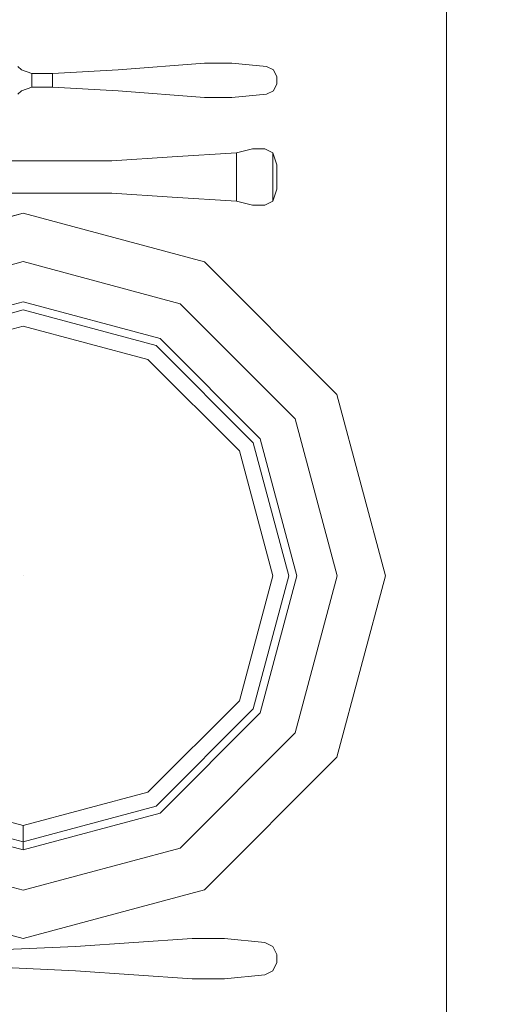
# Model space of a CAD drawing. Units: inches. Extents: x 375 to 1122, y 27 to 1069.
# Tile 63 of 155: x 739.72 to 747.02, y 296.54 to 311.59. Entities that reach past the tile are written whole.
import ezdxf

# ---------------------------------------------------------------- set-up
doc = ezdxf.new("R2010")
doc.units = ezdxf.units.IN
doc.layers.add('A-ANNO-DIMS', color=2, linetype='Continuous', lineweight=18)
doc.layers.add('Furniture', color=30, linetype='Continuous', lineweight=18)
doc.styles.get("Standard").update_dxf_attribs({"font": 'arial.ttf'})
doc.dimstyles.new('ISO-25', dxfattribs={"dimtxt": 12, "dimasz": 2.5, "dimexe": 1.5, "dimexo": 1.5, "dimtad": 1, "dimdec": 1, "dimlunit": 3, "dimtxsty": 'Standard', "dimblk": 'ARCHTICK', "dimcen": 2.5, "dimadec": 0, "dimazin": 0, "dimtfac": 1, "dimtdec": 1, "dimtmove": 0, "dimatfit": 3, "dimfxl": 1.5, "dimfxlon": 1, "dimarcsym": 0})

# ---------------------------------------------------------------- blocks, each defined once
blk = doc.blocks.new('A$C403C54AD')
blk.add_line((0.83575, 1.53256, -0.0006), (1.99923, 1.53256, -0.0006))
at = {"linetype": 'ByBlock'}
for points, invisible_edges in [([(1.0802, 1.50922, -0.02349), (1.0802, 1.49075, -0.02349), (1.02018, 1.47466, -0.02349), (1.01094, 1.49066, -0.02349)], 5), ([(1.0802, 1.47535, -0.03734), (1.0802, 1.50922, -0.02811), (1.01094, 1.49066, -0.02811), (1.02787, 1.46133, -0.03734)], 5), ([(1.14947, 1.49066, -0.02349), (1.14023, 1.47466, -0.02349), (1.0802, 1.49075, -0.02349), (1.0802, 1.50922, -0.02349)], 5), ([(1.13254, 1.46133, -0.03734), (1.14947, 1.49066, -0.02811), (1.0802, 1.50922, -0.02811), (1.0802, 1.47535, -0.03734)], 5), ([(1.01094, 1.49066, -0.02349), (1.02018, 1.47466, -0.02349), (0.97623, 1.43072, -0.02349), (0.96024, 1.43995, -0.02349)], 5), ([(1.02787, 1.46133, -0.03734), (1.01094, 1.49066, -0.02811), (0.96024, 1.43995, -0.02811), (0.98956, 1.42302, -0.03734)], 5), ([(1.0802, 1.49075, -0.02349), (1.0802, 1.47228, -0.02965), (1.02941, 1.45867, -0.02965), (1.02018, 1.47466, -0.02349)], 5), ([(1.14023, 1.47466, -0.02349), (1.131, 1.45867, -0.02965), (1.0802, 1.47228, -0.02965), (1.0802, 1.49075, -0.02349)], 5), ([(1.17085, 1.42302, -0.03734), (1.20017, 1.43995, -0.02811), (1.14947, 1.49066, -0.02811), (1.13254, 1.46133, -0.03734)], 5), ([(1.20017, 1.43995, -0.02349), (1.18418, 1.43072, -0.02349), (1.14023, 1.47466, -0.02349), (1.14947, 1.49066, -0.02349)], 5), ([(1.02018, 1.47466, -0.02349), (1.02941, 1.45867, -0.02965), (0.99223, 1.42148, -0.02965), (0.97623, 1.43072, -0.02349)], 5), ([(1.0802, 1.46612, -0.04658), (1.0802, 1.47535, -0.03734), (1.02787, 1.46133, -0.03734), (1.03249, 1.45333, -0.04658)], 5), ([(1.12792, 1.45333, -0.04658), (1.13254, 1.46133, -0.03734), (1.0802, 1.47535, -0.03734), (1.0802, 1.46612, -0.04658)], 5), ([(1.18418, 1.43072, -0.02349), (1.16818, 1.42148, -0.02965), (1.131, 1.45867, -0.02965), (1.14023, 1.47466, -0.02349)], 5), ([(1.0802, 1.47228, -0.02965), (1.0802, 1.37069, -0.02965), (1.0802, 1.37069, -0.02965), (1.02941, 1.45867, -0.02965)], 5), ([(1.131, 1.45867, -0.02965), (1.0802, 1.37069, -0.02965), (1.0802, 1.37069, -0.02965), (1.0802, 1.47228, -0.02965)], 5), ([(1.03249, 1.45333, -0.04658), (1.02787, 1.46133, -0.03734), (0.98956, 1.42302, -0.03734), (0.99756, 1.4184, -0.04658)], 5), ([(1.16285, 1.4184, -0.04658), (1.17085, 1.42302, -0.03734), (1.13254, 1.46133, -0.03734), (1.12792, 1.45333, -0.04658)], 5), ([(1.02941, 1.45867, -0.02965), (1.0802, 1.37069, -0.02965), (1.0802, 1.37069, -0.02965), (0.99223, 1.42148, -0.02965)], 5), ([(1.16818, 1.42148, -0.02965), (1.0802, 1.37069, -0.02965), (1.0802, 1.37069, -0.02965), (1.131, 1.45867, -0.02965)], 5), ([(0.96024, 1.43995, -0.02349), (0.97623, 1.43072, -0.02349), (0.96015, 1.37069, -0.02349), (0.94168, 1.37069, -0.02349)], 5), ([(0.98956, 1.42302, -0.03734), (0.96024, 1.43995, -0.02811), (0.94168, 1.37069, -0.02811), (0.97554, 1.37069, -0.03734)], 5), ([(1.18487, 1.37069, -0.03734), (1.21873, 1.37069, -0.02811), (1.20017, 1.43995, -0.02811), (1.17085, 1.42302, -0.03734)], 5), ([(1.21873, 1.37069, -0.02349), (1.20026, 1.37069, -0.02349), (1.18418, 1.43072, -0.02349), (1.20017, 1.43995, -0.02349)], 5), ([(0.97623, 1.43072, -0.02349), (0.99223, 1.42148, -0.02965), (0.97862, 1.37069, -0.02965), (0.96015, 1.37069, -0.02349)], 5), ([(1.20026, 1.37069, -0.02349), (1.18179, 1.37069, -0.02965), (1.16818, 1.42148, -0.02965), (1.18418, 1.43072, -0.02349)], 5), ([(0.99756, 1.4184, -0.04658), (0.98956, 1.42302, -0.03734), (0.97554, 1.37069, -0.03734), (0.98477, 1.37069, -0.04658)], 5), ([(1.17563, 1.37069, -0.04658), (1.18487, 1.37069, -0.03734), (1.17085, 1.42302, -0.03734), (1.16285, 1.4184, -0.04658)], 4), ([(0.99223, 1.42148, -0.02965), (1.0802, 1.37069, -0.02965), (1.0802, 1.37069, -0.02965), (0.97862, 1.37069, -0.02965)], 5), ([(1.18179, 1.37069, -0.02965), (1.0802, 1.37069, -0.02965), (1.0802, 1.37069, -0.02965), (1.16818, 1.42148, -0.02965)], 5), ([(0.94168, 1.37069, -0.02349), (0.96015, 1.37069, -0.02349), (0.97623, 1.31066, -0.02349), (0.96024, 1.30143, -0.02349)], 5), ([(0.97554, 1.37069, -0.03734), (0.94168, 1.37069, -0.02811), (0.96024, 1.30143, -0.02811), (0.98956, 1.31836, -0.03734)], 5), ([(0.96015, 1.37069, -0.02349), (0.97862, 1.37069, -0.02965), (0.99223, 1.3199, -0.02965), (0.97623, 1.31066, -0.02349)], 5), ([(0.98477, 1.37069, -0.04658), (0.97554, 1.37069, -0.03734), (0.98956, 1.31836, -0.03734), (0.99756, 1.32297, -0.04658)], 5), ([(0.97862, 1.37069, -0.02965), (1.0802, 1.37069, -0.02965), (1.0802, 1.37069, -0.02965), (0.99223, 1.3199, -0.02965)], 5), ([(0.99223, 1.3199, -0.02965), (1.0802, 1.37069, -0.02965), (1.0802, 1.37069, -0.02965), (1.02941, 1.28271, -0.02965)], 5), ([(1.02941, 1.28271, -0.02965), (1.0802, 1.37069, -0.02965), (1.0802, 1.37069, -0.02965), (1.0802, 1.2691, -0.02965)], 5), ([(1.0802, 1.2691, -0.02965), (1.0802, 1.37069, -0.02965), (1.0802, 1.37069, -0.02965), (1.131, 1.28271, -0.02965)], 5), ([(1.16818, 1.3199, -0.02965), (1.0802, 1.37069, -0.02965), (1.0802, 1.37069, -0.02965), (1.18179, 1.37069, -0.02965)], 5), ([(1.131, 1.28271, -0.02965), (1.0802, 1.37069, -0.02965), (1.0802, 1.37069, -0.02965), (1.16818, 1.3199, -0.02965)], 5), ([(1.18418, 1.31066, -0.02349), (1.16818, 1.3199, -0.02965), (1.18179, 1.37069, -0.02965), (1.20026, 1.37069, -0.02349)], 5), ([(1.17085, 1.31836, -0.03734), (1.20017, 1.30143, -0.02811), (1.21873, 1.37069, -0.02811), (1.18487, 1.37069, -0.03734)], 5), ([(1.20017, 1.30143, -0.02349), (1.18418, 1.31066, -0.02349), (1.20026, 1.37069, -0.02349), (1.21873, 1.37069, -0.02349)], 5)]:
    blk.add_3dface(points, dxfattribs=dict(at, invisible_edges=invisible_edges))
for points in [[(1.0802, 1.50922, -0.02811), (1.0802, 1.50922, -0.02349), (1.01094, 1.49066, -0.02349), (1.01094, 1.49066, -0.02811)], [(1.14947, 1.49066, -0.02811), (1.14947, 1.49066, -0.02349), (1.0802, 1.50922, -0.02349), (1.0802, 1.50922, -0.02811)], [(1.01094, 1.49066, -0.02811), (1.01094, 1.49066, -0.02349), (0.96024, 1.43995, -0.02349), (0.96024, 1.43995, -0.02811)], [(1.20017, 1.43995, -0.02811), (1.20017, 1.43995, -0.02349), (1.14947, 1.49066, -0.02349), (1.14947, 1.49066, -0.02811)], [(0.96024, 1.43995, -0.02811), (0.96024, 1.43995, -0.02349), (0.94168, 1.37069, -0.02349), (0.94168, 1.37069, -0.02811)], [(1.21873, 1.37069, -0.02811), (1.21873, 1.37069, -0.02349), (1.20017, 1.43995, -0.02349), (1.20017, 1.43995, -0.02811)], [(0.94168, 1.37069, -0.02811), (0.94168, 1.37069, -0.02349), (0.96024, 1.30143, -0.02349), (0.96024, 1.30143, -0.02811)], [(1.16285, 1.32297, -0.04658), (1.17085, 1.31836, -0.03734), (1.18487, 1.37069, -0.03734), (1.17563, 1.37069, -0.04658)], [(1.20017, 1.30143, -0.02811), (1.20017, 1.30143, -0.02349), (1.21873, 1.37069, -0.02349), (1.21873, 1.37069, -0.02811)]]:
    blk.add_3dface(points, dxfattribs=at)
for points, invisible_edges in [([(0.8922, 1.46766, -0.04251), (0.88956, 1.46766, -0.04251), (0.88693, 1.46634, -0.04237), (0.89484, 1.46634, -0.04237)], 4), ([(0.8922, 1.46766, -0.04605), (0.88956, 1.46766, -0.04605), (0.88693, 1.46634, -0.04634), (0.89484, 1.46634, -0.04634)], 4), ([(1.22797, 1.46766, -0.03413), (1.22489, 1.46766, -0.03413), (1.22181, 1.46612, -0.03397), (1.23105, 1.46612, -0.03397)], 4), ([(1.22797, 1.46766, -0.03827), (1.22489, 1.46766, -0.03827), (1.22181, 1.46612, -0.0386), (1.23105, 1.46612, -0.0386)], 4), ([(0.89616, 1.4637, -0.04257), (0.88561, 1.4637, -0.04257), (0.88429, 1.45051, -0.0426), (0.89748, 1.45051, -0.0426)], 5), ([(0.89616, 1.4637, -0.04655), (0.88561, 1.4637, -0.04655), (0.88429, 1.45051, -0.04658), (0.89748, 1.45051, -0.04658)], 5), ([(0.88693, 1.46634, -0.04237), (0.89484, 1.46634, -0.04237), (0.89616, 1.4637, -0.04257), (0.88561, 1.4637, -0.04257)], 5), ([(0.88693, 1.46634, -0.04634), (0.89484, 1.46634, -0.04634), (0.89616, 1.4637, -0.04655), (0.88561, 1.4637, -0.04655)], 5), ([(0.91705, 1.46304, -0.03581), (0.9386, 1.46304, -0.03581), (0.93706, 1.46612, -0.03734), (0.91859, 1.46612, -0.03734)], 1), ([(0.91705, 1.46304, -0.04504), (0.9386, 1.46304, -0.04504), (0.93706, 1.46612, -0.0435), (0.91859, 1.46612, -0.0435)], 1), ([(1.22181, 1.46612, -0.03397), (1.23105, 1.46612, -0.03397), (1.23258, 1.46304, -0.03421), (1.22027, 1.46304, -0.03421)], 5), ([(1.22181, 1.46612, -0.0386), (1.23105, 1.46612, -0.0386), (1.23258, 1.46304, -0.03884), (1.22027, 1.46304, -0.03884)], 5), ([(0.9386, 1.45842, -0.03427), (0.91705, 1.45842, -0.03427), (0.91705, 1.46304, -0.03581), (0.9386, 1.46304, -0.03581)], 5), ([(0.9386, 1.45842, -0.04658), (0.91705, 1.45842, -0.04658), (0.91705, 1.46304, -0.04504), (0.9386, 1.46304, -0.04504)], 5), ([(1.23258, 1.46304, -0.03421), (1.22027, 1.46304, -0.03421), (1.21873, 1.44765, -0.03425), (1.23412, 1.44765, -0.03425)], 5), ([(1.23258, 1.46304, -0.03884), (1.22027, 1.46304, -0.03884), (1.21873, 1.44765, -0.03888), (1.23412, 1.44765, -0.03888)], 5), ([(0.91859, 1.45227, -0.03581), (0.93706, 1.45227, -0.03581), (0.9386, 1.45842, -0.03427), (0.91705, 1.45842, -0.03427)], 4), ([(0.91859, 1.45227, -0.04504), (0.93706, 1.45227, -0.04504), (0.9386, 1.45842, -0.04658), (0.91705, 1.45842, -0.04658)], 4), ([(0.93552, 1.42764, -0.03427), (0.92013, 1.42764, -0.03427), (0.91859, 1.45227, -0.03581), (0.93706, 1.45227, -0.03581)], 1), ([(0.93552, 1.42764, -0.04658), (0.92013, 1.42764, -0.04658), (0.91859, 1.45227, -0.04504), (0.93706, 1.45227, -0.04504)], 1), ([(0.88429, 1.45051, -0.0426), (0.89748, 1.45051, -0.0426), (0.89748, 1.43995, -0.04232), (0.88429, 1.43995, -0.04232)], 5), ([(0.88429, 1.45051, -0.04658), (0.89748, 1.45051, -0.04658), (0.89748, 1.43995, -0.0463), (0.88429, 1.43995, -0.0463)], 5), ([(1.21873, 1.44765, -0.03425), (1.23412, 1.44765, -0.03425), (1.23412, 1.43534, -0.03392), (1.21873, 1.43534, -0.03392)], 5), ([(1.21873, 1.44765, -0.03888), (1.23412, 1.44765, -0.03888), (1.23412, 1.43534, -0.03855), (1.21873, 1.43534, -0.03855)], 5), ([(0.89748, 1.43995, -0.0463), (0.88429, 1.43995, -0.0463), (0.88693, 1.40697, -0.04292), (0.89484, 1.40697, -0.04292)], 5), ([(0.88429, 1.43995, -0.0463), (0.88429, 1.43995, -0.04232), (0.88693, 1.40697, -0.04028), (0.88693, 1.40697, -0.04292)], 4), ([(0.89748, 1.43995, -0.04232), (0.88429, 1.43995, -0.04232), (0.88693, 1.40697, -0.04028), (0.89484, 1.40697, -0.04028)], 5), ([(0.89484, 1.40697, -0.04292), (0.89484, 1.40697, -0.04028), (0.89748, 1.43995, -0.04232), (0.89748, 1.43995, -0.0463)], 1), ([(1.23412, 1.43534, -0.03392), (1.21873, 1.43534, -0.03392), (1.22181, 1.3907, -0.03153), (1.23105, 1.3907, -0.03153)], 5), ([(1.23412, 1.43534, -0.03855), (1.21873, 1.43534, -0.03855), (1.22181, 1.3907, -0.03461), (1.23105, 1.3907, -0.03461)], 5), ([(1.21873, 1.43534, -0.03855), (1.21873, 1.43534, -0.03392), (1.22181, 1.3907, -0.03153), (1.22181, 1.3907, -0.03461)], 4), ([(1.23105, 1.3907, -0.03461), (1.23105, 1.3907, -0.03153), (1.23412, 1.43534, -0.03392), (1.23412, 1.43534, -0.03855)], 1), ([(0.92167, 1.40455, -0.03427), (0.93398, 1.40455, -0.03427), (0.93552, 1.42764, -0.03427), (0.92013, 1.42764, -0.03427)], 5), ([(0.92167, 1.40455, -0.04658), (0.93398, 1.40455, -0.04658), (0.93552, 1.42764, -0.04658), (0.92013, 1.42764, -0.04658)], 5), ([(0.88693, 1.40697, -0.04028), (0.89484, 1.40697, -0.04028), (0.89352, 1.3819, -0.03779), (0.88825, 1.3819, -0.03779)], 1), ([(0.88693, 1.40697, -0.04028), (0.88693, 1.40697, -0.04292), (0.88825, 1.3819, -0.04001), (0.88825, 1.3819, -0.03779)], 5), ([(0.88693, 1.40697, -0.04292), (0.89484, 1.40697, -0.04292), (0.89352, 1.3819, -0.04001), (0.88825, 1.3819, -0.04001)], 1), ([(0.89352, 1.3819, -0.03779), (0.89352, 1.3819, -0.04001), (0.89484, 1.40697, -0.04292), (0.89484, 1.40697, -0.04028)], 5), ([(0.93398, 1.36607, -0.03581), (0.92167, 1.36607, -0.03581), (0.92167, 1.40455, -0.03427), (0.93398, 1.40455, -0.03427)], 4), ([(0.93398, 1.36607, -0.04504), (0.92167, 1.36607, -0.04504), (0.92167, 1.40455, -0.04658), (0.93398, 1.40455, -0.04658)], 4), ([(1.22181, 1.3907, -0.03153), (1.23105, 1.3907, -0.03153), (1.22951, 1.3553, -0.02863), (1.22335, 1.3553, -0.02863)], 1), ([(1.22181, 1.3907, -0.03153), (1.22181, 1.3907, -0.03461), (1.22335, 1.3553, -0.03122), (1.22335, 1.3553, -0.02863)], 5), ([(1.22181, 1.3907, -0.03461), (1.23105, 1.3907, -0.03461), (1.22951, 1.3553, -0.03122), (1.22335, 1.3553, -0.03122)], 1), ([(1.22951, 1.3553, -0.02863), (1.22951, 1.3553, -0.03122), (1.23105, 1.3907, -0.03461), (1.23105, 1.3907, -0.03153)], 5), ([(0.88825, 1.3819, -0.04001), (0.88825, 1.3819, -0.03779), (0.88825, 1.37399, -0.03842), (0.88825, 1.37399, -0.04064)], 5), ([(0.89352, 1.37399, -0.04064), (0.89352, 1.37399, -0.03842), (0.89352, 1.3819, -0.03779), (0.89352, 1.3819, -0.04001)], 5), ([(0.88825, 1.37399, -0.03842), (0.89352, 1.37399, -0.03842), (0.89484, 1.37003, -0.04027), (0.88693, 1.37003, -0.04027)], 4), ([(0.88825, 1.37399, -0.03842), (0.88825, 1.37399, -0.04064), (0.88693, 1.37003, -0.04236), (0.88693, 1.37003, -0.04027)], 5), ([(0.88825, 1.37399, -0.04064), (0.89352, 1.37399, -0.04064), (0.89484, 1.37003, -0.04236), (0.88693, 1.37003, -0.04236)], 4), ([(0.89352, 1.37399, -0.04064), (0.89352, 1.37399, -0.03842), (0.89484, 1.37003, -0.04027), (0.89484, 1.37003, -0.04236)], 5), ([(0.89484, 1.37003, -0.04027), (0.88693, 1.37003, -0.04027), (0.88561, 1.3687, -0.041), (0.89616, 1.3687, -0.041)], 5), ([(0.89484, 1.37003, -0.04236), (0.88693, 1.37003, -0.04236), (0.88561, 1.3687, -0.04315), (0.89616, 1.3687, -0.04315)], 5), ([(0.88693, 1.37003, -0.04236), (0.88693, 1.37003, -0.04027), (0.88561, 1.3687, -0.041), (0.88561, 1.3687, -0.04315)], 1), ([(0.89484, 1.37003, -0.04027), (0.89484, 1.37003, -0.04236), (0.89616, 1.3687, -0.04315), (0.89616, 1.3687, -0.041)], 1)]:
    blk.add_3dface(points, dxfattribs=dict(invisible_edges=invisible_edges))
for points in [[(0.88956, 1.46766, -0.04605), (0.88956, 1.46766, -0.04251), (0.88693, 1.46634, -0.04237), (0.88693, 1.46634, -0.04634)], [(0.8922, 1.46766, -0.04251), (0.8922, 1.46766, -0.04605), (0.88956, 1.46766, -0.04605), (0.88956, 1.46766, -0.04251)], [(0.89484, 1.46634, -0.04634), (0.89484, 1.46634, -0.04237), (0.8922, 1.46766, -0.04251), (0.8922, 1.46766, -0.04605)], [(0.93706, 1.46612, -0.03734), (0.91859, 1.46612, -0.03734), (0.92321, 1.46766, -0.04042), (0.93244, 1.46766, -0.04042)], [(0.92321, 1.46766, -0.04042), (0.92321, 1.46766, -0.04042), (0.91859, 1.46612, -0.03734), (0.91859, 1.46612, -0.0435)], [(0.93706, 1.46612, -0.0435), (0.91859, 1.46612, -0.0435), (0.92321, 1.46766, -0.04042), (0.93244, 1.46766, -0.04042)], [(0.93706, 1.46612, -0.03734), (0.93706, 1.46612, -0.0435), (0.93244, 1.46766, -0.04042)], [(1.22489, 1.46766, -0.03827), (1.22489, 1.46766, -0.03413), (1.22181, 1.46612, -0.03397), (1.22181, 1.46612, -0.0386)], [(1.22797, 1.46766, -0.03413), (1.22797, 1.46766, -0.03827), (1.22489, 1.46766, -0.03827), (1.22489, 1.46766, -0.03413)], [(1.23105, 1.46612, -0.0386), (1.23105, 1.46612, -0.03397), (1.22797, 1.46766, -0.03413), (1.22797, 1.46766, -0.03827)], [(0.88561, 1.4637, -0.04655), (0.88561, 1.4637, -0.04257), (0.88429, 1.45051, -0.0426), (0.88429, 1.45051, -0.04658)], [(0.88693, 1.46634, -0.04237), (0.88693, 1.46634, -0.04634), (0.88561, 1.4637, -0.04655), (0.88561, 1.4637, -0.04257)], [(0.89616, 1.4637, -0.04257), (0.89616, 1.4637, -0.04655), (0.89484, 1.46634, -0.04634), (0.89484, 1.46634, -0.04237)], [(0.89748, 1.45051, -0.04658), (0.89748, 1.45051, -0.0426), (0.89616, 1.4637, -0.04257), (0.89616, 1.4637, -0.04655)], [(0.91859, 1.46612, -0.03734), (0.91859, 1.46612, -0.0435), (0.91705, 1.46304, -0.04504), (0.91705, 1.46304, -0.03581)], [(0.9386, 1.46304, -0.04504), (0.9386, 1.46304, -0.03581), (0.93706, 1.46612, -0.03734), (0.93706, 1.46612, -0.0435)], [(1.22181, 1.46612, -0.03397), (1.22181, 1.46612, -0.0386), (1.22027, 1.46304, -0.03884), (1.22027, 1.46304, -0.03421)], [(1.23258, 1.46304, -0.03421), (1.23258, 1.46304, -0.03884), (1.23105, 1.46612, -0.0386), (1.23105, 1.46612, -0.03397)], [(0.91705, 1.46304, -0.03581), (0.91705, 1.46304, -0.04504), (0.91705, 1.45842, -0.04658), (0.91705, 1.45842, -0.03427)], [(0.9386, 1.45842, -0.03427), (0.9386, 1.45842, -0.04658), (0.9386, 1.46304, -0.04504), (0.9386, 1.46304, -0.03581)], [(1.22027, 1.46304, -0.03884), (1.22027, 1.46304, -0.03421), (1.21873, 1.44765, -0.03425), (1.21873, 1.44765, -0.03888)], [(1.23412, 1.44765, -0.03888), (1.23412, 1.44765, -0.03425), (1.23258, 1.46304, -0.03421), (1.23258, 1.46304, -0.03884)], [(0.91705, 1.45842, -0.04658), (0.91705, 1.45842, -0.03427), (0.91859, 1.45227, -0.03581), (0.91859, 1.45227, -0.04504)], [(0.93706, 1.45227, -0.04504), (0.93706, 1.45227, -0.03581), (0.9386, 1.45842, -0.03427), (0.9386, 1.45842, -0.04658)], [(0.91859, 1.45227, -0.03581), (0.91859, 1.45227, -0.04504), (0.92013, 1.42764, -0.04658), (0.92013, 1.42764, -0.03427)], [(0.93552, 1.42764, -0.03427), (0.93552, 1.42764, -0.04658), (0.93706, 1.45227, -0.04504), (0.93706, 1.45227, -0.03581)], [(0.88429, 1.45051, -0.0426), (0.88429, 1.45051, -0.04658), (0.88429, 1.43995, -0.0463), (0.88429, 1.43995, -0.04232)], [(0.89748, 1.43995, -0.04232), (0.89748, 1.43995, -0.0463), (0.89748, 1.45051, -0.04658), (0.89748, 1.45051, -0.0426)], [(1.21873, 1.44765, -0.03425), (1.21873, 1.44765, -0.03888), (1.21873, 1.43534, -0.03855), (1.21873, 1.43534, -0.03392)], [(1.23412, 1.43534, -0.03392), (1.23412, 1.43534, -0.03855), (1.23412, 1.44765, -0.03888), (1.23412, 1.44765, -0.03425)], [(0.92013, 1.42764, -0.04658), (0.92013, 1.42764, -0.03427), (0.92167, 1.40455, -0.03427), (0.92167, 1.40455, -0.04658)], [(0.93398, 1.40455, -0.04658), (0.93398, 1.40455, -0.03427), (0.93552, 1.42764, -0.03427), (0.93552, 1.42764, -0.04658)], [(0.92167, 1.40455, -0.03427), (0.92167, 1.40455, -0.04658), (0.92167, 1.36607, -0.04504), (0.92167, 1.36607, -0.03581)], [(0.93398, 1.36607, -0.03581), (0.93398, 1.36607, -0.04504), (0.93398, 1.40455, -0.04658), (0.93398, 1.40455, -0.03427)], [(0.89352, 1.3819, -0.04001), (0.88825, 1.3819, -0.04001), (0.88825, 1.37399, -0.04064), (0.89352, 1.37399, -0.04064)], [(0.89352, 1.3819, -0.03779), (0.88825, 1.3819, -0.03779), (0.88825, 1.37399, -0.03842), (0.89352, 1.37399, -0.03842)]]:
    blk.add_3dface(points)
blk = doc.blocks.new('_ArchTick')
at = {"color": 0, "linetype": 'ByBlock', "const_width": 0.15}
blk.add_lwpolyline([(-0.5, -0.5), (0.5, 0.5)], dxfattribs=at)
blk = doc.blocks.new('*D94')
at = {"layer": 'A-ANNO-DIMS', "color": 0, "lineweight": -2, "transparency": 16777216}
for p, q in [((734.007, 117.528), (734.007, 114.528)), ((773.007, 117.528), (773.007, 114.528)), ((734.007, 116.028), (773.007, 116.028))]:
    blk.add_line(p, q, dxfattribs=at)
at = {"layer": 'Defpoints', "color": 0, "transparency": 16777216}
for p in [(734.007, 667.528), (773.007, 667.528), (773.007, 116.028)]:
    blk.add_point(p, dxfattribs=at)
at = {"layer": 'A-ANNO-DIMS', "color": 0, "lineweight": -2, "transparency": 16777216, "xscale": 2.5, "yscale": 2.5, "zscale": 2.5, "rotation": 180}
blk.add_blockref('_ArchTick', (734.007, 116.028), dxfattribs=at)
at = {"layer": 'A-ANNO-DIMS', "color": 0, "lineweight": -2, "transparency": 16777216, "xscale": 2.5, "yscale": 2.5, "zscale": 2.5}
blk.add_blockref('_ArchTick', (773.007, 116.028), dxfattribs=at)
at = {"layer": 'A-ANNO-DIMS', "color": 0, "transparency": 16777216, "insert": (753.507, 122.784), "char_height": 12, "attachment_point": 5}
blk.add_mtext('3\'-3"', dxfattribs=at)

msp = doc.modelspace()

# ---------------------------------------------------------------- block references
at = {"layer": 'Furniture', "xscale": 39.9918517141215, "yscale": 39.9918517141215, "zscale": 39.9918517141215, "rotation": 270}
msp.add_blockref('A$C403C54AD', (684.955, 346.287, 0.024), dxfattribs=at)

# ---------------------------------------------------------------- dimensions: what is measured, and where the dimension line sits
at = {"layer": 'A-ANNO-DIMS'}
dim = msp.add_linear_dim(base=(773.007, 116.028), p1=(734.007, 667.528), p2=(773.007, 667.528), dimstyle='ISO-25', override={"dimdec": 1, "dimlfac": 1, "dimrnd": 0, "dimzin": 1, "dimdsep": 46, "dimlunit": 4, "dimfrac": 2}, dxfattribs=at)
dim.commit()
dim.dimension.update_dxf_attribs({"geometry": '*D94', "text_midpoint": (753.507, 122.784)})

doc.saveas('drawing.dxf')
